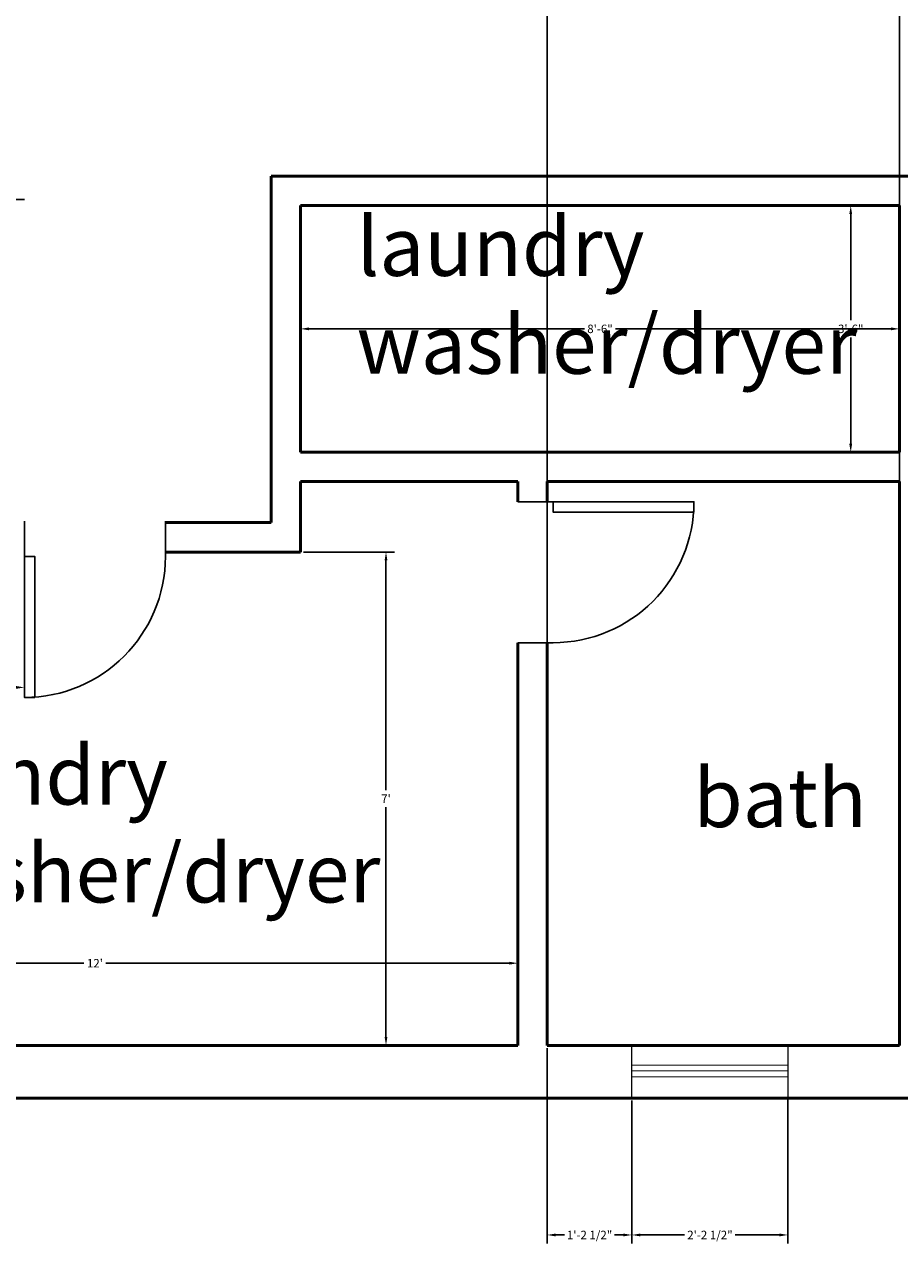
# Model space of a CAD drawing. Units: inches. Extents: x 325 to 804, y 366 to 834.
# Tile 3 of 6: x 496 to 645, y 366 to 574. Entities that reach past the tile are written whole.
import ezdxf

# ---------------------------------------------------------------- set-up
doc = ezdxf.new("R2010")
doc.units = ezdxf.units.IN
doc.header["$MEASUREMENT"] = 0
doc.layers.get('0').update_dxf_attribs({"color": 4})
for name, color, linetype, lineweight in [('A-ANNO-DIMS', 2, 'Continuous', 18), ('A-AREA-IDEN', 7, 'Continuous', 25), ('A-WALL', 7, 'Continuous', 50), ('door', 10, 'Continuous', 25), ('window', 3, 'Continuous', 18)]:
    doc.layers.add(name, color=color, linetype=linetype, lineweight=lineweight)
doc.styles.get("Standard").update_dxf_attribs({"font": 'arial.ttf'})
doc.dimstyles.get("Standard").update_dxf_attribs({"dimscale": 8, "dimtxt": 0.18, "dimasz": 0.18, "dimexe": 0.18, "dimexo": 0.0625, "dimgap": 0.09, "dimtad": 0, "dimtih": 1, "dimtoh": 1, "dimdec": 0, "dimzin": 0, "dimdsep": 46, "dimlunit": 3, "dimtxsty": 'Standard', "dimcen": 0.09, "dimadec": 0, "dimazin": 0, "dimtfac": 1, "dimtdec": 0, "dimtofl": 0, "dimtmove": 0, "dimatfit": 3, "dimfxl": 1, "dimtolj": 1, "dimtzin": 0, "dimarcsym": 0})

# ---------------------------------------------------------------- blocks, each defined once
blk = doc.blocks.new('*U3')
for p, q in [((0, 0), (0, -6)), ((40, 0), (40, -6))]:
    blk.add_line(p, q)
blk.add_lwpolyline([(0, 0), (0, 40), (1.75, 40), (1.75, 0)], close=True)
blk.add_arc((0, 0), 40, 0, 90)
blk = doc.blocks.new('*U6')
for p, q in [((-24, 0), (-24, 6)), ((0, 0), (0, 6))]:
    blk.add_line(p, q)
blk.add_lwpolyline([(0, 0), (0, -24), (-1.75, -24), (-1.75, 0)], close=True)
blk.add_arc((0, 0), 24, 180, 270)
blk = doc.blocks.new('*U7')
for p, q in [((0, 0), (0, -6)), ((-24, 0), (-24, -6))]:
    blk.add_line(p, q)
blk.add_lwpolyline([(0, 0), (0, 24), (-1.75, 24), (-1.75, 0)], close=True)
blk.add_arc((0, 0), 24, 90, 180)
blk = doc.blocks.new('*D17')
at = {"layer": 'A-ANNO-DIMS', "color": 0, "lineweight": -2, "transparency": 16777216}
for p, q in [((436.47, 417.88), (436.47, 413.09)), ((580.47, 417.88), (580.47, 413.09)), ((437.91, 414.53), (506.6, 414.53)), ((579.03, 414.53), (510.35, 414.53))]:
    blk.add_line(p, q, dxfattribs=at)
at = {"layer": 'A-ANNO-DIMS', "color": 0, "transparency": 16777216}
for points in [[(437.91, 414.77), (437.91, 414.29), (436.47, 414.53)], [(579.03, 414.77), (579.03, 414.29), (580.47, 414.53)]]:
    blk.add_solid(points, dxfattribs=at)
at = {"layer": 'Defpoints', "color": 0, "transparency": 16777216}
for p in [(436.47, 418.38), (580.47, 418.38), (580.47, 414.53)]:
    blk.add_point(p, dxfattribs=at)
at = {"layer": 'A-ANNO-DIMS', "color": 0, "transparency": 16777216, "insert": (508.47, 414.53), "char_height": 1.44, "attachment_point": 5}
blk.add_mtext("\\A1;12'", dxfattribs=at)
blk = doc.blocks.new('*D18')
at = {"layer": 'A-ANNO-DIMS', "color": 0, "lineweight": -2, "transparency": 16777216}
for p, q in [((543.97, 484.54), (559.47, 484.54)), ((558.03, 483.1), (558.03, 443.98)), ((558.03, 401.98), (558.03, 441.1)), ((543.97, 400.54), (559.47, 400.54))]:
    blk.add_line(p, q, dxfattribs=at)
at = {"layer": 'A-ANNO-DIMS', "color": 0, "transparency": 16777216}
for points in [[(557.79, 483.1), (558.27, 483.1), (558.03, 484.54)], [(557.79, 401.98), (558.27, 401.98), (558.03, 400.54)]]:
    blk.add_solid(points, dxfattribs=at)
at = {"layer": 'Defpoints', "color": 0, "transparency": 16777216}
for p in [(543.47, 484.54), (543.47, 400.54), (558.03, 400.54)]:
    blk.add_point(p, dxfattribs=at)
at = {"layer": 'A-ANNO-DIMS', "color": 0, "transparency": 16777216, "insert": (558.03, 442.54), "char_height": 1.44, "attachment_point": 5}
blk.add_mtext("\\A1;7'", dxfattribs=at)
blk = doc.blocks.new('*D19')
at = {"layer": 'A-ANNO-DIMS', "color": 0, "lineweight": -2, "transparency": 16777216}
for p, q in [((543.47, 523.04), (543.47, 523.98)), ((645.47, 523.04), (645.47, 523.98)), ((544.91, 522.54), (591.84, 522.54)), ((644.03, 522.54), (597.11, 522.54))]:
    blk.add_line(p, q, dxfattribs=at)
at = {"layer": 'A-ANNO-DIMS', "color": 0, "transparency": 16777216}
for points in [[(544.91, 522.78), (544.91, 522.3), (543.47, 522.54)], [(644.03, 522.78), (644.03, 522.3), (645.47, 522.54)]]:
    blk.add_solid(points, dxfattribs=at)
at = {"layer": 'Defpoints', "color": 0, "transparency": 16777216}
for p in [(543.47, 522.54), (645.47, 522.54), (645.47, 522.54)]:
    blk.add_point(p, dxfattribs=at)
at = {"layer": 'A-ANNO-DIMS', "color": 0, "transparency": 16777216, "insert": (594.47, 522.54), "char_height": 1.44, "attachment_point": 5}
blk.add_mtext('\\A1;8\'-6"', dxfattribs=at)
blk = doc.blocks.new('*D20')
at = {"layer": 'A-ANNO-DIMS', "color": 0, "lineweight": -2, "transparency": 16777216}
for p, q in [((644.97, 543.54), (635.72, 543.54)), ((637.16, 542.1), (637.16, 523.99)), ((637.16, 502.98), (637.16, 521.08)), ((644.97, 501.54), (635.72, 501.54))]:
    blk.add_line(p, q, dxfattribs=at)
at = {"layer": 'A-ANNO-DIMS', "color": 0, "transparency": 16777216}
for points in [[(636.92, 542.1), (637.4, 542.1), (637.16, 543.54)], [(636.92, 502.98), (637.4, 502.98), (637.16, 501.54)]]:
    blk.add_solid(points, dxfattribs=at)
at = {"layer": 'Defpoints', "color": 0, "transparency": 16777216}
for p in [(645.47, 543.54), (637.16, 501.54), (645.47, 501.54)]:
    blk.add_point(p, dxfattribs=at)
at = {"layer": 'A-ANNO-DIMS', "color": 0, "transparency": 16777216, "insert": (637.16, 522.54), "char_height": 1.44, "attachment_point": 5}
blk.add_mtext('\\A1;3\'-6"', dxfattribs=at)
blk = doc.blocks.new('*D33')
at = {"layer": 'A-ANNO-DIMS', "color": 0, "lineweight": -2, "transparency": 16777216}
for p, q in [((599.9, 391.18), (599.9, 366.82)), ((626.47, 391.24), (626.47, 366.82)), ((601.34, 368.26), (608.86, 368.26)), ((625.03, 368.26), (617.51, 368.26))]:
    blk.add_line(p, q, dxfattribs=at)
at = {"layer": 'A-ANNO-DIMS', "color": 0, "transparency": 16777216}
for points in [[(601.34, 368.5), (601.34, 368.02), (599.9, 368.26)], [(625.03, 368.5), (625.03, 368.02), (626.47, 368.26)]]:
    blk.add_solid(points, dxfattribs=at)
at = {"layer": 'Defpoints', "color": 0, "transparency": 16777216}
for p in [(599.9, 391.68), (626.47, 391.74), (626.47, 368.26)]:
    blk.add_point(p, dxfattribs=at)
at = {"layer": 'A-ANNO-DIMS', "color": 0, "transparency": 16777216, "insert": (613.19, 368.26), "char_height": 1.44, "attachment_point": 5}
blk.add_mtext('\\A1;2\'-2 1/2"', dxfattribs=at)
blk = doc.blocks.new('*D34')
at = {"layer": 'A-ANNO-DIMS', "color": 0, "lineweight": -2, "transparency": 16777216}
for p, q in [((585.47, 400.04), (585.47, 366.82)), ((599.9, 391.18), (599.9, 366.82)), ((586.91, 368.26), (588.44, 368.26)), ((598.46, 368.26), (596.93, 368.26))]:
    blk.add_line(p, q, dxfattribs=at)
at = {"layer": 'A-ANNO-DIMS', "color": 0, "transparency": 16777216}
for points in [[(586.91, 368.5), (586.91, 368.02), (585.47, 368.26)], [(598.46, 368.5), (598.46, 368.02), (599.9, 368.26)]]:
    blk.add_solid(points, dxfattribs=at)
at = {"layer": 'Defpoints', "color": 0, "transparency": 16777216}
for p in [(585.47, 400.54), (599.9, 391.68), (599.9, 368.26)]:
    blk.add_point(p, dxfattribs=at)
at = {"layer": 'A-ANNO-DIMS', "color": 0, "transparency": 16777216, "insert": (592.69, 368.26), "char_height": 1.44, "attachment_point": 5}
blk.add_mtext('\\A1;1\'-2 1/2"', dxfattribs=at)
blk = doc.blocks.new('*D38')
at = {"layer": 'A-ANNO-DIMS', "color": 0, "lineweight": -2, "transparency": 16777216}
for p, q in [((585.47, 401.04), (585.47, 786.03)), ((645.47, 401.04), (645.47, 786.03)), ((586.91, 784.59), (612.84, 784.59)), ((644.03, 784.59), (618.11, 784.59))]:
    blk.add_line(p, q, dxfattribs=at)
at = {"layer": 'A-ANNO-DIMS', "color": 0, "transparency": 16777216}
for points in [[(586.91, 784.83), (586.91, 784.35), (585.47, 784.59)], [(644.03, 784.83), (644.03, 784.35), (645.47, 784.59)]]:
    blk.add_solid(points, dxfattribs=at)
at = {"layer": 'Defpoints', "color": 0, "transparency": 16777216}
for p in [(645.47, 784.59), (585.47, 400.54), (645.47, 400.54)]:
    blk.add_point(p, dxfattribs=at)
at = {"layer": 'A-ANNO-DIMS', "color": 0, "transparency": 16777216, "insert": (615.47, 784.59), "char_height": 1.44, "attachment_point": 5}
blk.add_mtext('\\A1;5\'-0"', dxfattribs=at)
blk = doc.blocks.new('*D46')
at = {"layer": 'A-ANNO-DIMS', "color": 0, "lineweight": -2, "transparency": 16777216}
for p, q in [((436.47, 484.04), (436.47, 460.05)), ((496.47, 484.04), (496.47, 460.05)), ((437.91, 461.49), (463.84, 461.49)), ((495.03, 461.49), (469.11, 461.49))]:
    blk.add_line(p, q, dxfattribs=at)
at = {"layer": 'A-ANNO-DIMS', "color": 0, "transparency": 16777216}
for points in [[(437.91, 461.73), (437.91, 461.25), (436.47, 461.49)], [(495.03, 461.73), (495.03, 461.25), (496.47, 461.49)]]:
    blk.add_solid(points, dxfattribs=at)
at = {"layer": 'Defpoints', "color": 0, "transparency": 16777216}
for p in [(436.47, 484.54), (496.47, 484.54), (436.47, 461.49)]:
    blk.add_point(p, dxfattribs=at)
at = {"layer": 'A-ANNO-DIMS', "color": 0, "transparency": 16777216, "insert": (466.47, 461.49), "char_height": 1.44, "attachment_point": 5}
blk.add_mtext('\\A1;5\'-0"', dxfattribs=at)

msp = doc.modelspace()

# ---------------------------------------------------------------- linework, layer by layer
at = {"layer": 'A-WALL'}
for p, q in [((538.47, 548.54), (650.47, 548.54)), ((538.47, 489.54), (538.47, 548.54)), ((543.47, 543.54), (645.47, 543.54)), ((543.47, 501.54), (543.47, 543.54)), ((645.47, 501.54), (645.47, 543.54)), ((543.47, 501.54), (580.47, 501.54)), ((580.47, 501.54), (645.47, 501.54)), ((543.47, 484.54), (543.47, 496.54)), ((543.47, 496.54), (580.47, 496.54)), ((580.47, 496.54), (580.47, 493.1)), ((585.47, 496.54), (645.47, 496.54)), ((585.47, 493.1), (585.47, 496.54)), ((645.47, 400.54), (645.47, 496.54)), ((520.47, 489.54), (538.47, 489.54)), ((520.47, 484.54), (543.47, 484.54)), ((580.47, 469.1), (580.47, 400.54)), ((585.47, 400.54), (585.47, 469.1)), ((436.47, 400.54), (580.47, 400.54)), ((585.47, 400.54), (645.47, 400.54)), ((350.47, 391.54), (774.47, 391.54))]:
    msp.add_line(p, q, dxfattribs=at)
at = {"layer": 'door'}
msp.add_line((491.47, 544.54), (496.47, 544.54), dxfattribs=at)
at = {"layer": 'window'}
for p, q in [((599.9, 391.68), (599.9, 400.68)), ((626.47, 400.74), (626.47, 391.74)), ((599.9, 397.18), (626.47, 397.24)), ((599.9, 396.18), (626.47, 396.24)), ((599.9, 395.18), (626.47, 395.24))]:
    msp.add_line(p, q, dxfattribs=at)

# ---------------------------------------------------------------- block references
at = {"layer": 'door', "rotation": 90}
msp.add_blockref('*U3', (490.47, 544.54), dxfattribs=at)
at = {"layer": 'door', "xscale": -1, "rotation": 270}
msp.add_blockref('*U7', (586.47, 493.1), dxfattribs=at)
at = {"layer": 'door', "xscale": -1}
msp.add_blockref('*U6', (496.47, 483.78), dxfattribs=at)

# ---------------------------------------------------------------- texts
at = {"layer": 'A-AREA-IDEN', "char_height": 10, "attachment_point": 1}
for s, width, heights, insert in [('laundry washer/dryer', 25.6907, [0], (553.02, 541.56)), ('laundry washer/dryer', 25.6907, [0], (471.88, 451.54)), ('bath', 20.8578, [0.203], (610.34, 447.7))]:
    msp.add_mtext_dynamic_manual_height_columns(s, width=width, gutter_width=1, heights=heights, dxfattribs=dict(at, insert=insert))

# ---------------------------------------------------------------- dimensions: what is measured, and where the dimension line sits
at = {"layer": 'A-ANNO-DIMS'}
for base, p1, p2, override, picture, middle in [((645.47, 784.59), (585.47, 400.54), (645.47, 400.54), {"dimdec": 1, "dimlfac": 1, "dimrnd": 0, "dimzin": 1, "dimdsep": 46, "dimlunit": 4, "dimfrac": 2}, '*D38', (615.47, 784.59)), ((645.47, 522.54), (543.47, 522.54), (645.47, 522.54), {"dimclrd": 0, "dimclre": 0, "dimclrt": 0}, '*D19', (594.47, 522.54)), ((580.47, 414.53), (436.47, 418.38), (580.47, 418.38), {"dimclrd": 0, "dimclre": 0, "dimclrt": 0}, '*D17', (508.47, 414.53)), ((599.9, 368.26), (585.47, 400.54), (599.9, 391.68), {"dimdec": 1, "dimlfac": 1, "dimrnd": 0, "dimzin": 1, "dimdsep": 46, "dimlunit": 4, "dimfrac": 2}, '*D34', (592.69, 368.26)), ((626.47, 368.26), (599.9, 391.68), (626.47, 391.74), {"dimdec": 1, "dimlfac": 1, "dimrnd": 0, "dimzin": 1, "dimdsep": 46, "dimlunit": 4, "dimfrac": 2}, '*D33', (613.19, 368.26))]:
    dim = msp.add_linear_dim(base=base, p1=p1, p2=p2, dimstyle='Standard', override=override, dxfattribs=at)
    dim.commit()
    dim.dimension.update_dxf_attribs({"geometry": picture, "text_midpoint": middle})
for base, p1, p2, angle, override, picture, middle in [((637.16, 501.54), (645.47, 543.54), (645.47, 501.54), 90, {"dimclrd": 0, "dimclre": 0, "dimclrt": 0}, '*D20', (637.16, 522.54)), ((436.47, 461.49), (496.47, 484.54), (436.47, 484.54), 180, {"dimdec": 1, "dimlfac": 1, "dimrnd": 0, "dimzin": 1, "dimdsep": 46, "dimlunit": 4, "dimfrac": 2}, '*D46', (466.47, 461.49)), ((558.03, 400.54), (543.47, 484.54), (543.47, 400.54), 90, {"dimclrd": 0, "dimclre": 0, "dimclrt": 0}, '*D18', (558.03, 442.54))]:
    dim = msp.add_linear_dim(base=base, p1=p1, p2=p2, angle=angle, dimstyle='Standard', override=override, dxfattribs=at)
    dim.commit()
    dim.dimension.update_dxf_attribs({"geometry": picture, "text_midpoint": middle})

doc.saveas('drawing.dxf')
